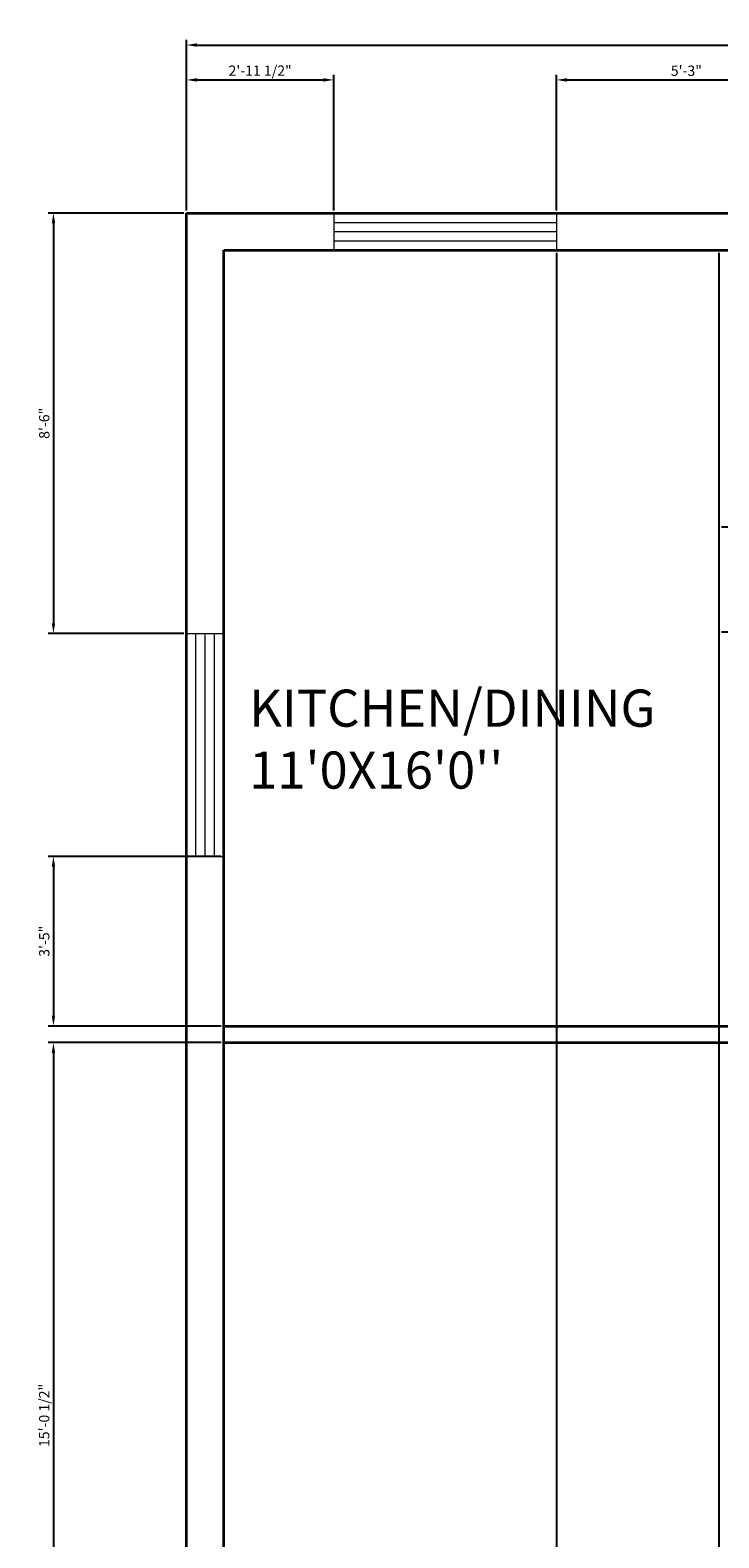
# Model space of a CAD drawing. Units: inches. Extents: x 2572 to 3021, y 1553 to 2232.
# Tile 2 of 3: x 2572 to 2739, y 1866 to 2232. Entities that reach past the tile are written whole.
import ezdxf

# ---------------------------------------------------------------- set-up
doc = ezdxf.new("R2010")
doc.units = ezdxf.units.IN
for name, color, linetype, lineweight in [('A-ANNO-DIMS', 2, 'Continuous', 18), ('A-AREA-IDEN', 7, 'Continuous', 25), ('A-GLAZ', 4, 'Continuous', 18), ('A-WALL', 7, 'Continuous', 35)]:
    doc.layers.add(name, color=color, linetype=linetype, lineweight=lineweight)
doc.styles.get("Standard").update_dxf_attribs({"font": 'arial.ttf'})
doc.dimstyles.new('ISO-25', dxfattribs={"dimtxt": 2.5, "dimasz": 2.5, "dimexe": 1.25, "dimexo": 0.625, "dimtad": 1, "dimdec": 1, "dimlunit": 3, "dimtxsty": 'Standard', "dimcen": 2.5, "dimadec": 0, "dimazin": 0, "dimtfac": 1, "dimtdec": 1, "dimtmove": 0, "dimatfit": 3, "dimfxl": 1, "dimarcsym": 0})

# ---------------------------------------------------------------- blocks, each defined once
blk = doc.blocks.new('Window - Wood Frame 36 in. Wide plan')
for p, q in [((0, 6), (0, 0)), ((36, 6), (36, 0)), ((0, 4.5), (36, 4.5)), ((0, 3), (36, 3)), ((0, 1.5), (36, 1.5))]:
    blk.add_line(p, q)
blk = doc.blocks.new('*D7')
at = {"layer": 'A-ANNO-DIMS', "color": 0, "lineweight": -2, "transparency": 16777216}
for p, q in [((2610.18, 2188), (2610.18, 2229.34)), ((2970.18, 2188), (2970.18, 2229.34)), ((2612.68, 2228.09), (2967.68, 2228.09))]:
    blk.add_line(p, q, dxfattribs=at)
at = {"layer": 'A-ANNO-DIMS', "color": 0, "transparency": 16777216}
for points in [[(2612.68, 2228.5), (2612.68, 2227.67), (2610.18, 2228.09)], [(2967.68, 2228.5), (2967.68, 2227.67), (2970.18, 2228.09)]]:
    blk.add_solid(points, dxfattribs=at)
at = {"layer": 'Defpoints', "color": 0, "transparency": 16777216}
for p in [(2970.18, 2228.09), (2610.18, 2187.37), (2970.18, 2187.37)]:
    blk.add_point(p, dxfattribs=at)
at = {"layer": 'A-ANNO-DIMS', "color": 0, "transparency": 16777216, "insert": (2790.18, 2229.99), "char_height": 2.5, "attachment_point": 5}
blk.add_mtext("30'", dxfattribs=at)
blk = doc.blocks.new('*D20')
at = {"layer": 'A-ANNO-DIMS', "color": 0, "lineweight": -2, "transparency": 16777216}
for p, q in [((2610.18, 2188), (2610.18, 2220.88)), ((2612.68, 2219.63), (2643.35, 2219.63)), ((2645.85, 2188), (2645.85, 2220.88))]:
    blk.add_line(p, q, dxfattribs=at)
at = {"layer": 'A-ANNO-DIMS', "color": 0, "transparency": 16777216}
for points in [[(2612.68, 2220.05), (2612.68, 2219.21), (2610.18, 2219.63)], [(2643.35, 2220.05), (2643.35, 2219.21), (2645.85, 2219.63)]]:
    blk.add_solid(points, dxfattribs=at)
at = {"layer": 'Defpoints', "color": 0, "transparency": 16777216}
for p in [(2645.85, 2219.63), (2610.18, 2187.37), (2645.85, 2187.37)]:
    blk.add_point(p, dxfattribs=at)
at = {"layer": 'A-ANNO-DIMS', "color": 0, "transparency": 16777216, "insert": (2628.01, 2221.55), "char_height": 2.5, "attachment_point": 5}
blk.add_mtext('2\'-11 1/2"', dxfattribs=at)
blk = doc.blocks.new('*D21')
at = {"layer": 'A-ANNO-DIMS', "color": 0, "lineweight": -2, "transparency": 16777216}
for p, q in [((2699.85, 2188), (2699.85, 2220.88)), ((2702.35, 2219.63), (2760.25, 2219.63)), ((2762.75, 2188), (2762.75, 2220.88))]:
    blk.add_line(p, q, dxfattribs=at)
at = {"layer": 'A-ANNO-DIMS', "color": 0, "transparency": 16777216}
for points in [[(2702.35, 2220.05), (2702.35, 2219.21), (2699.85, 2219.63)], [(2760.25, 2220.05), (2760.25, 2219.21), (2762.75, 2219.63)]]:
    blk.add_solid(points, dxfattribs=at)
at = {"layer": 'Defpoints', "color": 0, "transparency": 16777216}
for p in [(2762.75, 2219.63), (2699.85, 2187.37), (2762.75, 2187.37)]:
    blk.add_point(p, dxfattribs=at)
at = {"layer": 'A-ANNO-DIMS', "color": 0, "transparency": 16777216, "insert": (2731.3, 2221.53), "char_height": 2.5, "attachment_point": 5}
blk.add_mtext('5\'-3"', dxfattribs=at)
blk = doc.blocks.new('*D23')
at = {"layer": 'A-ANNO-DIMS', "color": 0, "lineweight": -2, "transparency": 16777216}
for p, q in [((2609.55, 2187.37), (2576.67, 2187.37)), ((2577.92, 2184.87), (2577.92, 2088)), ((2609.55, 2085.5), (2576.67, 2085.5))]:
    blk.add_line(p, q, dxfattribs=at)
at = {"layer": 'A-ANNO-DIMS', "color": 0, "transparency": 16777216}
for points in [[(2577.51, 2184.87), (2578.34, 2184.87), (2577.92, 2187.37)], [(2577.51, 2088), (2578.34, 2088), (2577.92, 2085.5)]]:
    blk.add_solid(points, dxfattribs=at)
at = {"layer": 'Defpoints', "color": 0, "transparency": 16777216}
for p in [(2610.18, 2187.37), (2577.92, 2085.5), (2610.18, 2085.5)]:
    blk.add_point(p, dxfattribs=at)
at = {"layer": 'A-ANNO-DIMS', "color": 0, "transparency": 16777216, "insert": (2576.02, 2136.43), "char_height": 2.5, "attachment_point": 5, "rotation": 90}
blk.add_mtext('8\'-6"', dxfattribs=at)
blk = doc.blocks.new('*D24')
at = {"layer": 'A-ANNO-DIMS', "color": 0, "lineweight": -2, "transparency": 16777216}
for p, q in [((2618.55, 1986.37), (2576.67, 1986.37)), ((2577.92, 1983.87), (2577.92, 1808.21)), ((2609.55, 1805.71), (2576.67, 1805.71))]:
    blk.add_line(p, q, dxfattribs=at)
at = {"layer": 'A-ANNO-DIMS', "color": 0, "transparency": 16777216}
for points in [[(2577.51, 1983.87), (2578.34, 1983.87), (2577.92, 1986.37)], [(2577.51, 1808.21), (2578.34, 1808.21), (2577.92, 1805.71)]]:
    blk.add_solid(points, dxfattribs=at)
at = {"layer": 'Defpoints', "color": 0, "transparency": 16777216}
for p in [(2619.18, 1986.37), (2577.92, 1805.71), (2610.18, 1805.71)]:
    blk.add_point(p, dxfattribs=at)
at = {"layer": 'A-ANNO-DIMS', "color": 0, "transparency": 16777216, "insert": (2576, 1896.04), "char_height": 2.5, "attachment_point": 5, "rotation": 90}
blk.add_mtext('15\'-0 1/2"', dxfattribs=at)
blk = doc.blocks.new('*D34')
at = {"layer": 'A-ANNO-DIMS', "color": 0, "lineweight": -2, "transparency": 16777216}
for p, q in [((2739.8, 2111.37), (3003.68, 2111.37)), ((3002.43, 2108.87), (3002.43, 2088.44)), ((2739.8, 2085.94), (3003.68, 2085.94))]:
    blk.add_line(p, q, dxfattribs=at)
at = {"layer": 'A-ANNO-DIMS', "color": 0, "transparency": 16777216}
for points in [[(3002.02, 2108.87), (3002.85, 2108.87), (3002.43, 2111.37)], [(3002.02, 2088.44), (3002.85, 2088.44), (3002.43, 2085.94)]]:
    blk.add_solid(points, dxfattribs=at)
at = {"layer": 'Defpoints', "color": 0, "transparency": 16777216}
for p in [(2739.18, 2111.37), (2739.18, 2085.94), (3002.43, 2085.94)]:
    blk.add_point(p, dxfattribs=at)
at = {"layer": 'A-ANNO-DIMS', "color": 0, "transparency": 16777216, "insert": (3000.51, 2098.66), "char_height": 2.5, "attachment_point": 5, "rotation": 90}
blk.add_mtext('2\'-1 1/2"', dxfattribs=at)
blk = doc.blocks.new('*D38')
at = {"layer": 'A-ANNO-DIMS', "color": 0, "lineweight": -2, "transparency": 16777216}
for p, q in [((2699.85, 2177.75), (2699.85, 1553.87)), ((2739.18, 2177.75), (2739.18, 1553.87)), ((2736.68, 1555.12), (2702.35, 1555.12))]:
    blk.add_line(p, q, dxfattribs=at)
at = {"layer": 'A-ANNO-DIMS', "color": 0, "transparency": 16777216}
for points in [[(2702.35, 1555.54), (2702.35, 1554.7), (2699.85, 1555.12)], [(2736.68, 1555.54), (2736.68, 1554.7), (2739.18, 1555.12)]]:
    blk.add_solid(points, dxfattribs=at)
at = {"layer": 'Defpoints', "color": 0, "transparency": 16777216}
for p in [(2699.85, 2178.37), (2739.18, 2178.37), (2699.85, 1555.12)]:
    blk.add_point(p, dxfattribs=at)
at = {"layer": 'A-ANNO-DIMS', "color": 0, "transparency": 16777216, "insert": (2719.51, 1557.04), "char_height": 2.5, "attachment_point": 5}
blk.add_mtext('3\'-3 1/2"', dxfattribs=at)
blk = doc.blocks.new('*D40')
at = {"layer": 'A-ANNO-DIMS', "color": 0, "lineweight": -2, "transparency": 16777216}
for p, q in [((2618.55, 2031.5), (2576.67, 2031.5)), ((2577.92, 2029), (2577.92, 1992.87)), ((2618.55, 1990.37), (2576.67, 1990.37))]:
    blk.add_line(p, q, dxfattribs=at)
at = {"layer": 'A-ANNO-DIMS', "color": 0, "transparency": 16777216}
for points in [[(2577.51, 2029), (2578.34, 2029), (2577.92, 2031.5)], [(2577.51, 1992.87), (2578.34, 1992.87), (2577.92, 1990.37)]]:
    blk.add_solid(points, dxfattribs=at)
at = {"layer": 'Defpoints', "color": 0, "transparency": 16777216}
for p in [(2619.18, 2031.5), (2577.92, 1990.37), (2619.18, 1990.37)]:
    blk.add_point(p, dxfattribs=at)
at = {"layer": 'A-ANNO-DIMS', "color": 0, "transparency": 16777216, "insert": (2576.02, 2010.93), "char_height": 2.5, "attachment_point": 5, "rotation": 90}
blk.add_mtext('3\'-5"', dxfattribs=at)

msp = doc.modelspace()

# ---------------------------------------------------------------- linework, layer by layer
at = {"layer": 'A-WALL'}
for p, q in [((2610.18, 2187.37), (2970.18, 2187.37)), ((2610.18, 1587.37), (2610.18, 2187.37)), ((2619.18, 1592.85), (2619.18, 2178.37)), ((2619.18, 2178.37), (2961.18, 2178.37)), ((2619.18, 1990.37), (2743.18, 1990.37)), ((2619.18, 1986.37), (2743.18, 1986.37))]:
    msp.add_line(p, q, dxfattribs=at)

# ---------------------------------------------------------------- block references
at = {"layer": 'A-GLAZ', "xscale": 1.5, "yscale": 1.5, "zscale": 1.5}
msp.add_blockref('Window - Wood Frame 36 in. Wide plan', (2645.85, 2178.37), dxfattribs=at)
at = {"layer": 'A-GLAZ', "xscale": 1.5, "yscale": 1.5, "zscale": 1.5, "rotation": 90}
msp.add_blockref('Window - Wood Frame 36 in. Wide plan', (2619.18, 2031.5), dxfattribs=at)

# ---------------------------------------------------------------- texts
at = {"layer": 'A-AREA-IDEN', "insert": (2625.37, 2071.91), "char_height": 9, "attachment_point": 1}
msp.add_mtext_dynamic_manual_height_columns("\\pxt12;KITCHEN/DINING                     \\P\\ptz;11'0X16'0''", width=94.3643, gutter_width=12.5, heights=[0], dxfattribs=at)

# ---------------------------------------------------------------- dimensions: what is measured, and where the dimension line sits
at = {"layer": 'A-ANNO-DIMS'}
for base, p1, p2, override, picture, middle in [((2970.18, 2228.09), (2610.18, 2187.37), (2970.18, 2187.37), {"dimclrd": 0, "dimclre": 0, "dimclrt": 0}, '*D7', (2790.18, 2229.99)), ((2645.85, 2219.63), (2610.18, 2187.37), (2645.85, 2187.37), {"dimdec": 1, "dimlfac": 1, "dimrnd": 0, "dimzin": 1, "dimdsep": 46, "dimlunit": 4, "dimfrac": 2}, '*D20', (2628.01, 2221.55)), ((2762.75, 2219.63), (2699.85, 2187.37), (2762.75, 2187.37), {"dimdec": 1, "dimlfac": 1, "dimrnd": 0, "dimzin": 1, "dimdsep": 46, "dimlunit": 4, "dimfrac": 2}, '*D21', (2731.3, 2221.53)), ((2699.85, 1555.12), (2739.18, 2178.37), (2699.85, 2178.37), {"dimdec": 1, "dimlfac": 1, "dimrnd": 0, "dimzin": 1, "dimdsep": 46, "dimlunit": 4, "dimfrac": 2}, '*D38', (2719.51, 1557.04))]:
    dim = msp.add_linear_dim(base=base, p1=p1, p2=p2, dimstyle='ISO-25', override=override, dxfattribs=at)
    dim.commit()
    dim.dimension.update_dxf_attribs({"geometry": picture, "text_midpoint": middle})
for base, p1, p2, picture, middle in [((2577.92, 2085.5), (2610.18, 2187.37), (2610.18, 2085.5), '*D23', (2576.02, 2136.43)), ((3002.43, 2085.94), (2739.18, 2111.37), (2739.18, 2085.94), '*D34', (3000.51, 2098.66)), ((2577.92, 1990.37), (2619.18, 2031.5), (2619.18, 1990.37), '*D40', (2576.02, 2010.93)), ((2577.92, 1805.71), (2619.18, 1986.37), (2610.18, 1805.71), '*D24', (2576, 1896.04))]:
    dim = msp.add_linear_dim(base=base, p1=p1, p2=p2, angle=90, dimstyle='ISO-25', override={"dimdec": 1, "dimlfac": 1, "dimrnd": 0, "dimzin": 1, "dimdsep": 46, "dimlunit": 4, "dimfrac": 2}, dxfattribs=at)
    dim.commit()
    dim.dimension.update_dxf_attribs({"geometry": picture, "text_midpoint": middle})

doc.saveas('drawing.dxf')
